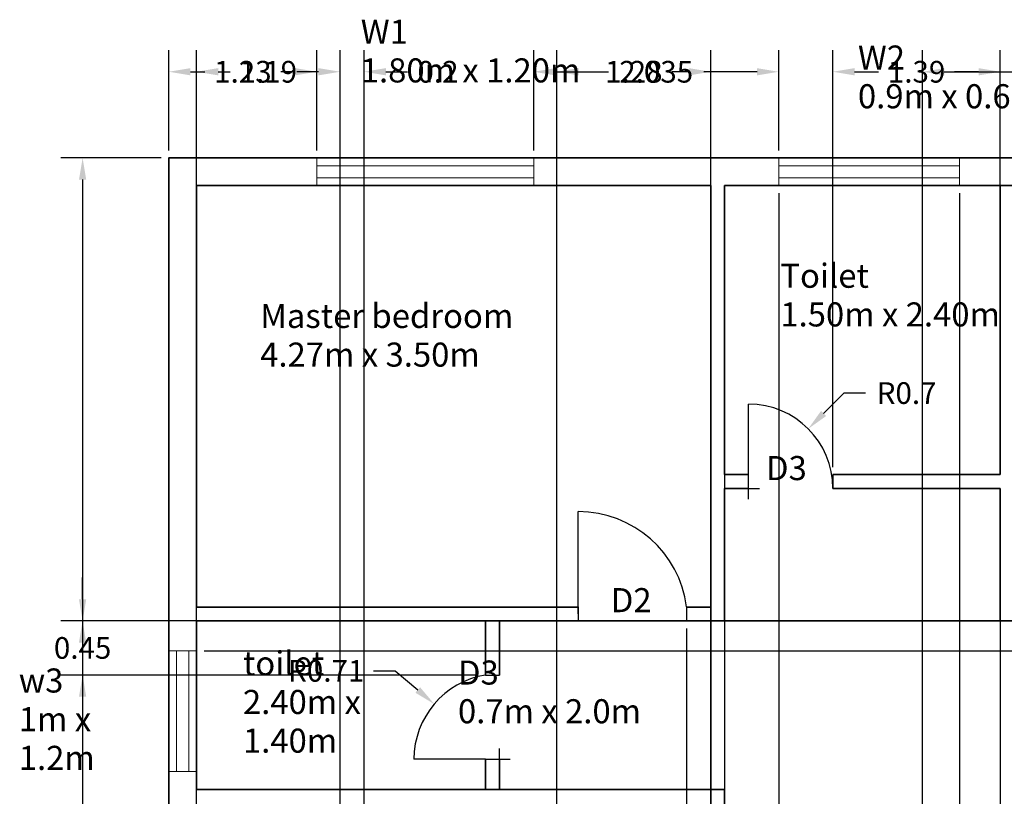
# Model space of a CAD drawing. Units: metres. Extents: x 1585.4 to 1599.4, y 2063.3 to 2076.9.
# Tile 2 of 3: x 1585.7 to 1593.9, y 2070.4 to 2076.9. Entities that reach past the tile are written whole.
import ezdxf

# ---------------------------------------------------------------- set-up
doc = ezdxf.new("R2010")
doc.units = ezdxf.units.M
for name, color, linetype, lineweight in [('A-ANNO-DIMS', 2, 'Continuous', 18), ('A-ANNO-TEXT', 7, 'Continuous', 18), ('A-AREA-IDEN', 7, 'Continuous', 18), ('A-DOOR', 3, 'Continuous', 25), ('A-GLAZ', 4, 'Continuous', 18), ('A-WALL', 7, 'Continuous', 35)]:
    doc.layers.add(name, color=color, linetype=linetype, lineweight=lineweight)
doc.styles.get("Standard").update_dxf_attribs({"font": 'arial.ttf'})
doc.dimstyles.get("Standard").update_dxf_attribs({"dimtxt": 0.18, "dimasz": 0.18, "dimexe": 0.18, "dimexo": 0.0625, "dimgap": 0.09, "dimtad": 0, "dimtih": 1, "dimtoh": 1, "dimdec": 4, "dimzin": 0, "dimdsep": 46, "dimtxsty": 'Standard', "dimcen": 0.09, "dimadec": 0, "dimazin": 0, "dimtfac": 1, "dimtdec": 4, "dimtofl": 0, "dimtmove": 0, "dimatfit": 3, "dimfxl": 1, "dimtolj": 1, "dimtzin": 0, "dimarcsym": 0})

# ---------------------------------------------------------------- blocks, each defined once
blk = doc.blocks.new('WIN-FRAME-1800')
for p, q in [((0, 0), (0, 0.23)), ((0, 0.23), (1.8, 0.23)), ((1.8, 0.23), (1.8, 0))]:
    blk.add_line(p, q)
blk = doc.blocks.new('WIN-FRAME-1500')
for p, q in [((0, 0), (0, 0.23)), ((0, 0.23), (1.5, 0.23)), ((1.5, 0.23), (1.5, 0))]:
    blk.add_line(p, q)
blk = doc.blocks.new('WIN-FRAME-1000')
for p, q in [((0, 0), (0, 1)), ((0, 1), (0.23, 1)), ((0.23, 0), (0, 0))]:
    blk.add_line(p, q)
blk = doc.blocks.new('DOOR-900-JAMBS-SWING')
for p, q in [((0.7923, 0.9), (0.9073, 0.9)), ((0.7923, 0), (0.9073, 0))]:
    blk.add_line(p, q)
blk.add_arc((0.9073, 0), 0.9073, 97.28167, 180)
blk = doc.blocks.new('*D7')
at = {"layer": 'A-ANNO-DIMS', "color": 0, "lineweight": -2, "transparency": 16777216}
for p, q in [((1586.8683, 2075.7088), (1586.0348, 2075.7088)), ((1586.2148, 2075.5288), (1586.2148, 2070.1307)), ((1586.2148, 2064.3688), (1586.2148, 2069.7669)), ((1591.4833, 2064.1888), (1586.0348, 2064.1888))]:
    blk.add_line(p, q, dxfattribs=at)
at = {"layer": 'A-ANNO-DIMS', "color": 0, "transparency": 16777216}
for points in [[(1586.1848, 2075.5288), (1586.2448, 2075.5288), (1586.2148, 2075.7088)], [(1586.1848, 2064.3688), (1586.2448, 2064.3688), (1586.2148, 2064.1888)]]:
    blk.add_solid(points, dxfattribs=at)
at = {"layer": 'Defpoints', "color": 0, "transparency": 16777216}
for p in [(1586.2148, 2075.7088), (1586.9308, 2075.7088), (1591.5458, 2064.1888)]:
    blk.add_point(p, dxfattribs=at)
at = {"layer": 'A-ANNO-DIMS', "color": 0, "transparency": 16777216, "insert": (1586.2148, 2069.9488), "char_height": 0.18, "attachment_point": 5}
blk.add_mtext('\\A1;11.52', dxfattribs=at)
blk = doc.blocks.new('*D8')
at = {"layer": 'A-ANNO-DIMS', "color": 0, "lineweight": -2, "transparency": 16777216}
for p, q in [((1590.1533, 2067.2463), (1590.1533, 2076.6048)), ((1591.4308, 2067.2463), (1591.4308, 2076.6048)), ((1590.3333, 2076.4248), (1590.4766, 2076.4248)), ((1591.2508, 2076.4248), (1591.1076, 2076.4248))]:
    blk.add_line(p, q, dxfattribs=at)
at = {"layer": 'A-ANNO-DIMS', "color": 0, "transparency": 16777216}
for points in [[(1590.3333, 2076.4548), (1590.3333, 2076.3948), (1590.1533, 2076.4248)], [(1591.2508, 2076.4548), (1591.2508, 2076.3948), (1591.4308, 2076.4248)]]:
    blk.add_solid(points, dxfattribs=at)
at = {"layer": 'Defpoints', "color": 0, "transparency": 16777216}
for p in [(1591.4308, 2076.4248), (1590.1533, 2067.1838), (1591.4308, 2067.1838)]:
    blk.add_point(p, dxfattribs=at)
at = {"layer": 'A-ANNO-DIMS', "color": 0, "transparency": 16777216, "insert": (1590.7921, 2076.4248), "char_height": 0.18, "attachment_point": 5}
blk.add_mtext('\\A1;1.28', dxfattribs=at)
blk = doc.blocks.new('*D11')
at = {"layer": 'A-ANNO-DIMS', "color": 0, "lineweight": -2, "transparency": 16777216}
for p, q in [((1586.9308, 2075.7713), (1586.9308, 2076.6048)), ((1588.1608, 2075.7713), (1588.1608, 2076.6048)), ((1587.1108, 2076.4248), (1587.2305, 2076.4248)), ((1587.9808, 2076.4248), (1587.8611, 2076.4248))]:
    blk.add_line(p, q, dxfattribs=at)
at = {"layer": 'A-ANNO-DIMS', "color": 0, "transparency": 16777216}
for points in [[(1587.1108, 2076.4548), (1587.1108, 2076.3948), (1586.9308, 2076.4248)], [(1587.9808, 2076.4548), (1587.9808, 2076.3948), (1588.1608, 2076.4248)]]:
    blk.add_solid(points, dxfattribs=at)
at = {"layer": 'Defpoints', "color": 0, "transparency": 16777216}
for p in [(1588.1608, 2076.4248), (1586.9308, 2075.7088), (1588.1608, 2075.7088)]:
    blk.add_point(p, dxfattribs=at)
at = {"layer": 'A-ANNO-DIMS', "color": 0, "transparency": 16777216, "insert": (1587.5458, 2076.4248), "char_height": 0.18, "attachment_point": 5}
blk.add_mtext('\\A1;1.23', dxfattribs=at)
blk = doc.blocks.new('*D12')
at = {"layer": 'A-ANNO-DIMS', "color": 0, "lineweight": -2, "transparency": 16777216}
for p, q in [((1589.9608, 2075.7713), (1589.9608, 2076.6048)), ((1591.9958, 2075.7713), (1591.9958, 2076.6048)), ((1590.1408, 2076.4248), (1590.5824, 2076.4248)), ((1591.8158, 2076.4248), (1591.3742, 2076.4248))]:
    blk.add_line(p, q, dxfattribs=at)
at = {"layer": 'A-ANNO-DIMS', "color": 0, "transparency": 16777216}
for points in [[(1590.1408, 2076.4548), (1590.1408, 2076.3948), (1589.9608, 2076.4248)], [(1591.8158, 2076.4548), (1591.8158, 2076.3948), (1591.9958, 2076.4248)]]:
    blk.add_solid(points, dxfattribs=at)
at = {"layer": 'Defpoints', "color": 0, "transparency": 16777216}
for p in [(1591.9958, 2076.4248), (1589.9608, 2075.7088), (1591.9958, 2075.7088)]:
    blk.add_point(p, dxfattribs=at)
at = {"layer": 'A-ANNO-DIMS', "color": 0, "transparency": 16777216, "insert": (1590.9783, 2076.4248), "char_height": 0.18, "attachment_point": 5}
blk.add_mtext('\\A1;2.035', dxfattribs=at)
blk = doc.blocks.new('*D13')
at = {"layer": 'A-ANNO-DIMS', "color": 0, "lineweight": -2, "transparency": 16777216}
for p, q in [((1591.9958, 2075.4163), (1591.9958, 2063.2928)), ((1593.4958, 2075.4163), (1593.4958, 2063.2928)), ((1592.1758, 2063.4728), (1592.4998, 2063.4728)), ((1593.3158, 2063.4728), (1592.9919, 2063.4728))]:
    blk.add_line(p, q, dxfattribs=at)
at = {"layer": 'A-ANNO-DIMS', "color": 0, "transparency": 16777216}
for points in [[(1592.1758, 2063.5028), (1592.1758, 2063.4428), (1591.9958, 2063.4728)], [(1593.3158, 2063.5028), (1593.3158, 2063.4428), (1593.4958, 2063.4728)]]:
    blk.add_solid(points, dxfattribs=at)
at = {"layer": 'Defpoints', "color": 0, "transparency": 16777216}
for p in [(1591.9958, 2075.4788), (1593.4958, 2075.4788), (1593.4958, 2063.4728)]:
    blk.add_point(p, dxfattribs=at)
at = {"layer": 'A-ANNO-DIMS', "color": 0, "transparency": 16777216, "insert": (1592.7458, 2063.4728), "char_height": 0.18, "attachment_point": 5}
blk.add_mtext('\\A1;1.5', dxfattribs=at)
blk = doc.blocks.new('*D21')
at = {"layer": 'A-ANNO-DIMS', "color": 0, "lineweight": -2, "transparency": 16777216}
for p, q in [((1598.1468, 2072.0438), (1598.1468, 2072.2238)), ((1587.2233, 2071.8638), (1598.3268, 2071.8638)), ((1587.2233, 2071.6138), (1598.3268, 2071.6138)), ((1598.1468, 2071.4338), (1598.1468, 2071.2538)), ((1598.1468, 2071.2538), (1597.9668, 2071.2538))]:
    blk.add_line(p, q, dxfattribs=at)
at = {"layer": 'A-ANNO-DIMS', "color": 0, "transparency": 16777216}
for points in [[(1598.1168, 2072.0438), (1598.1768, 2072.0438), (1598.1468, 2071.8638)], [(1598.1168, 2071.4338), (1598.1768, 2071.4338), (1598.1468, 2071.6138)]]:
    blk.add_solid(points, dxfattribs=at)
at = {"layer": 'Defpoints', "color": 0, "transparency": 16777216}
for p in [(1587.1608, 2071.8638), (1587.1608, 2071.6138), (1598.1468, 2071.6138)]:
    blk.add_point(p, dxfattribs=at)
at = {"layer": 'A-ANNO-DIMS', "color": 0, "transparency": 16777216, "insert": (1597.6424, 2071.2538), "char_height": 0.18, "attachment_point": 5}
blk.add_mtext('\\A1;0.25', dxfattribs=at)
blk = doc.blocks.new('*D22')
at = {"layer": 'A-ANNO-DIMS', "color": 0, "lineweight": -2, "transparency": 16777216}
for p, q in [((1591.4308, 2075.4163), (1591.4308, 2063.2928)), ((1591.5458, 2075.4163), (1591.5458, 2063.2928)), ((1591.2508, 2063.4728), (1591.0708, 2063.4728)), ((1591.7258, 2063.4728), (1591.9058, 2063.4728))]:
    blk.add_line(p, q, dxfattribs=at)
at = {"layer": 'A-ANNO-DIMS', "color": 0, "transparency": 16777216}
for points in [[(1591.2508, 2063.5028), (1591.2508, 2063.4428), (1591.4308, 2063.4728)], [(1591.7258, 2063.5028), (1591.7258, 2063.4428), (1591.5458, 2063.4728)]]:
    blk.add_solid(points, dxfattribs=at)
at = {"layer": 'Defpoints', "color": 0, "transparency": 16777216}
for p in [(1591.4308, 2075.4788), (1591.5458, 2075.4788), (1591.5458, 2063.4728)]:
    blk.add_point(p, dxfattribs=at)
at = {"layer": 'A-ANNO-DIMS', "color": 0, "transparency": 16777216, "insert": (1592.3002, 2063.4728), "char_height": 0.18, "attachment_point": 5}
blk.add_mtext('\\A1;0.115', dxfattribs=at)
blk = doc.blocks.new('*D23')
at = {"layer": 'A-ANNO-DIMS', "color": 0, "lineweight": -2, "transparency": 16777216}
for p, q in [((1591.5458, 2072.9013), (1591.5458, 2063.2928)), ((1593.8358, 2072.9013), (1593.8358, 2063.2928)), ((1591.7258, 2063.4728), (1592.3653, 2063.4728)), ((1593.6558, 2063.4728), (1593.0163, 2063.4728))]:
    blk.add_line(p, q, dxfattribs=at)
at = {"layer": 'A-ANNO-DIMS', "color": 0, "transparency": 16777216}
for points in [[(1591.7258, 2063.5028), (1591.7258, 2063.4428), (1591.5458, 2063.4728)], [(1593.6558, 2063.5028), (1593.6558, 2063.4428), (1593.8358, 2063.4728)]]:
    blk.add_solid(points, dxfattribs=at)
at = {"layer": 'Defpoints', "color": 0, "transparency": 16777216}
for p in [(1591.5458, 2072.9638), (1593.8358, 2072.9638), (1593.8358, 2063.4728)]:
    blk.add_point(p, dxfattribs=at)
at = {"layer": 'A-ANNO-DIMS', "color": 0, "transparency": 16777216, "insert": (1592.6908, 2063.4728), "char_height": 0.18, "attachment_point": 5}
blk.add_mtext('\\A1;2.29', dxfattribs=at)
blk = doc.blocks.new('*D26')
at = {"layer": 'A-ANNO-DIMS', "color": 0, "lineweight": -2, "transparency": 16777216}
for p, q in [((1593.1908, 2065.1163), (1593.1908, 2076.6048)), ((1597.2008, 2065.1163), (1597.2008, 2076.6048)), ((1593.3708, 2076.4248), (1594.8858, 2076.4248)), ((1597.0208, 2076.4248), (1595.5058, 2076.4248))]:
    blk.add_line(p, q, dxfattribs=at)
at = {"layer": 'A-ANNO-DIMS', "color": 0, "transparency": 16777216}
for points in [[(1593.3708, 2076.4548), (1593.3708, 2076.3948), (1593.1908, 2076.4248)], [(1597.0208, 2076.4548), (1597.0208, 2076.3948), (1597.2008, 2076.4248)]]:
    blk.add_solid(points, dxfattribs=at)
at = {"layer": 'Defpoints', "color": 0, "transparency": 16777216}
for p in [(1597.2008, 2076.4248), (1593.1908, 2065.0538), (1597.2008, 2065.0538)]:
    blk.add_point(p, dxfattribs=at)
at = {"layer": 'A-ANNO-DIMS', "color": 0, "transparency": 16777216, "insert": (1595.1958, 2076.4248), "char_height": 0.18, "attachment_point": 5}
blk.add_mtext('\\A1;4.01', dxfattribs=at)
blk = doc.blocks.new('*D27')
at = {"layer": 'A-ANNO-DIMS', "color": 0, "lineweight": -2, "transparency": 16777216}
for p, q in [((1587.1608, 2067.2463), (1587.1608, 2076.6048)), ((1588.3533, 2067.2463), (1588.3533, 2076.6048)), ((1587.3408, 2076.4248), (1587.4416, 2076.4248)), ((1588.1733, 2076.4248), (1588.0726, 2076.4248))]:
    blk.add_line(p, q, dxfattribs=at)
at = {"layer": 'A-ANNO-DIMS', "color": 0, "transparency": 16777216}
for points in [[(1587.3408, 2076.4548), (1587.3408, 2076.3948), (1587.1608, 2076.4248)], [(1588.1733, 2076.4548), (1588.1733, 2076.3948), (1588.3533, 2076.4248)]]:
    blk.add_solid(points, dxfattribs=at)
at = {"layer": 'Defpoints', "color": 0, "transparency": 16777216}
for p in [(1588.3533, 2076.4248), (1587.1608, 2067.1838), (1588.3533, 2067.1838)]:
    blk.add_point(p, dxfattribs=at)
at = {"layer": 'A-ANNO-DIMS', "color": 0, "transparency": 16777216, "insert": (1587.7571, 2076.4248), "char_height": 0.18, "attachment_point": 5}
blk.add_mtext('\\A1;1.19', dxfattribs=at)
blk = doc.blocks.new('*D28')
at = {"layer": 'A-ANNO-DIMS', "color": 0, "lineweight": -2, "transparency": 16777216}
for p, q in [((1588.3533, 2067.2463), (1588.3533, 2076.6048)), ((1588.5533, 2067.2463), (1588.5533, 2076.6048)), ((1588.1733, 2076.4248), (1587.9933, 2076.4248)), ((1588.7333, 2076.4248), (1588.9133, 2076.4248))]:
    blk.add_line(p, q, dxfattribs=at)
at = {"layer": 'A-ANNO-DIMS', "color": 0, "transparency": 16777216}
for points in [[(1588.1733, 2076.4548), (1588.1733, 2076.3948), (1588.3533, 2076.4248)], [(1588.7333, 2076.4548), (1588.7333, 2076.3948), (1588.5533, 2076.4248)]]:
    blk.add_solid(points, dxfattribs=at)
at = {"layer": 'Defpoints', "color": 0, "transparency": 16777216}
for p in [(1588.5533, 2076.4248), (1588.3533, 2067.1838), (1588.5533, 2067.1838)]:
    blk.add_point(p, dxfattribs=at)
at = {"layer": 'A-ANNO-DIMS', "color": 0, "transparency": 16777216, "insert": (1589.1663, 2076.4248), "char_height": 0.18, "attachment_point": 5}
blk.add_mtext('\\A1;0.2', dxfattribs=at)
blk = doc.blocks.new('*D31')
at = {"layer": 'A-ANNO-DIMS', "color": 0, "lineweight": -2, "transparency": 16777216}
for p, q in [((1593.8358, 2071.8013), (1593.8358, 2063.2928)), ((1594.1508, 2071.8013), (1594.1508, 2063.2928)), ((1593.6558, 2063.4728), (1593.4758, 2063.4728)), ((1594.3308, 2063.4728), (1594.5108, 2063.4728))]:
    blk.add_line(p, q, dxfattribs=at)
at = {"layer": 'A-ANNO-DIMS', "color": 0, "transparency": 16777216}
for points in [[(1593.6558, 2063.5028), (1593.6558, 2063.4428), (1593.8358, 2063.4728)], [(1594.3308, 2063.5028), (1594.3308, 2063.4428), (1594.1508, 2063.4728)]]:
    blk.add_solid(points, dxfattribs=at)
at = {"layer": 'Defpoints', "color": 0, "transparency": 16777216}
for p in [(1593.8358, 2071.8638), (1594.1508, 2071.8638), (1594.1508, 2063.4728)]:
    blk.add_point(p, dxfattribs=at)
at = {"layer": 'A-ANNO-DIMS', "color": 0, "transparency": 16777216, "insert": (1594.9052, 2063.4728), "char_height": 0.18, "attachment_point": 5}
blk.add_mtext('\\A1;0.315', dxfattribs=at)
blk = doc.blocks.new('*D32')
at = {"layer": 'A-ANNO-DIMS', "color": 0, "lineweight": -2, "transparency": 16777216}
for p, q in [((1591.4308, 2071.9163), (1591.4308, 2063.2928)), ((1591.2308, 2071.8013), (1591.2308, 2063.2928)), ((1591.0508, 2063.4728), (1590.8708, 2063.4728)), ((1591.6108, 2063.4728), (1591.7908, 2063.4728))]:
    blk.add_line(p, q, dxfattribs=at)
at = {"layer": 'A-ANNO-DIMS', "color": 0, "transparency": 16777216}
for points in [[(1591.0508, 2063.5028), (1591.0508, 2063.4428), (1591.2308, 2063.4728)], [(1591.6108, 2063.5028), (1591.6108, 2063.4428), (1591.4308, 2063.4728)]]:
    blk.add_solid(points, dxfattribs=at)
at = {"layer": 'Defpoints', "color": 0, "transparency": 16777216}
for p in [(1591.4308, 2071.9788), (1591.2308, 2071.8638), (1591.4308, 2063.4728)]:
    blk.add_point(p, dxfattribs=at)
at = {"layer": 'A-ANNO-DIMS', "color": 0, "transparency": 16777216, "insert": (1592.0438, 2063.4728), "char_height": 0.18, "attachment_point": 5}
blk.add_mtext('\\A1;0.2', dxfattribs=at)
blk = doc.blocks.new('*D34')
at = {"layer": 'A-ANNO-DIMS', "color": 0, "lineweight": -2, "transparency": 16777216}
for p, q in [((1592.4458, 2073.1413), (1592.4458, 2076.6048)), ((1593.8358, 2073.1413), (1593.8358, 2076.6048)), ((1592.6258, 2076.4248), (1592.8253, 2076.4248)), ((1593.6558, 2076.4248), (1593.4563, 2076.4248))]:
    blk.add_line(p, q, dxfattribs=at)
at = {"layer": 'A-ANNO-DIMS', "color": 0, "transparency": 16777216}
for points in [[(1592.6258, 2076.4548), (1592.6258, 2076.3948), (1592.4458, 2076.4248)], [(1593.6558, 2076.4548), (1593.6558, 2076.3948), (1593.8358, 2076.4248)]]:
    blk.add_solid(points, dxfattribs=at)
at = {"layer": 'Defpoints', "color": 0, "transparency": 16777216}
for p in [(1593.8358, 2076.4248), (1592.4458, 2073.0788), (1593.8358, 2073.0788)]:
    blk.add_point(p, dxfattribs=at)
at = {"layer": 'A-ANNO-DIMS', "color": 0, "transparency": 16777216, "insert": (1593.1408, 2076.4248), "char_height": 0.18, "attachment_point": 5}
blk.add_mtext('\\A1;1.39', dxfattribs=at)
blk = doc.blocks.new('*D35')
at = {"layer": 'A-ANNO-DIMS', "color": 0, "lineweight": -2, "transparency": 16777216}
for p, q in [((1586.214822, 2072.043841), (1586.214822, 2072.223841)), ((1589.498322, 2071.863841), (1586.034822, 2071.863841)), ((1589.498322, 2071.413841), (1586.034822, 2071.413841)), ((1586.214822, 2071.233841), (1586.214822, 2071.053841))]:
    blk.add_line(p, q, dxfattribs=at)
at = {"layer": 'A-ANNO-DIMS', "color": 0, "transparency": 16777216}
for points in [[(1586.184822, 2072.043841), (1586.244822, 2072.043841), (1586.214822, 2071.863841)], [(1586.184822, 2071.233841), (1586.244822, 2071.233841), (1586.214822, 2071.413841)]]:
    blk.add_solid(points, dxfattribs=at)
at = {"layer": 'Defpoints', "color": 0, "transparency": 16777216}
for p in [(1586.214822, 2071.863841), (1589.560822, 2071.863841), (1589.560822, 2071.413841)]:
    blk.add_point(p, dxfattribs=at)
at = {"layer": 'A-ANNO-DIMS', "color": 0, "transparency": 16777216, "insert": (1586.214822, 2071.638841), "char_height": 0.18, "attachment_point": 5}
blk.add_mtext('\\A1;0.45', dxfattribs=at)
blk = doc.blocks.new('*D36')
at = {"layer": 'A-ANNO-DIMS', "color": 0, "lineweight": -2, "transparency": 16777216}
for p, q in [((1591.5458, 2070.4013), (1591.5458, 2063.2928)), ((1597.2008, 2070.4598), (1597.2008, 2063.2928)), ((1591.7258, 2063.4728), (1593.9789, 2063.4728)), ((1597.0208, 2063.4728), (1594.7677, 2063.4728))]:
    blk.add_line(p, q, dxfattribs=at)
at = {"layer": 'A-ANNO-DIMS', "color": 0, "transparency": 16777216}
for points in [[(1591.7258, 2063.5028), (1591.7258, 2063.4428), (1591.5458, 2063.4728)], [(1597.0208, 2063.5028), (1597.0208, 2063.4428), (1597.2008, 2063.4728)]]:
    blk.add_solid(points, dxfattribs=at)
at = {"layer": 'Defpoints', "color": 0, "transparency": 16777216}
for p in [(1591.5458, 2070.4638), (1597.2008, 2070.5223), (1597.2008, 2063.4728)]:
    blk.add_point(p, dxfattribs=at)
at = {"layer": 'A-ANNO-DIMS', "color": 0, "transparency": 16777216, "insert": (1594.3733, 2063.4728), "char_height": 0.18, "attachment_point": 5}
blk.add_mtext('\\A1;5.655', dxfattribs=at)
blk = doc.blocks.new('*D37')
at = {"layer": 'A-ANNO-DIMS', "color": 0, "lineweight": -2, "transparency": 16777216}
for p, q in [((1597.1383, 2071.8638), (1586.0348, 2071.8638)), ((1586.2148, 2071.6838), (1586.2148, 2069.6)), ((1586.2148, 2067.1523), (1586.2148, 2069.2362)), ((1597.1383, 2066.9723), (1586.0348, 2066.9723))]:
    blk.add_line(p, q, dxfattribs=at)
at = {"layer": 'A-ANNO-DIMS', "color": 0, "transparency": 16777216}
for points in [[(1586.1848, 2071.6838), (1586.2448, 2071.6838), (1586.2148, 2071.8638)], [(1586.1848, 2067.1523), (1586.2448, 2067.1523), (1586.2148, 2066.9723)]]:
    blk.add_solid(points, dxfattribs=at)
at = {"layer": 'Defpoints', "color": 0, "transparency": 16777216}
for p in [(1586.2148, 2071.8638), (1597.2008, 2071.8638), (1597.2008, 2066.9723)]:
    blk.add_point(p, dxfattribs=at)
at = {"layer": 'A-ANNO-DIMS', "color": 0, "transparency": 16777216, "insert": (1586.2148, 2069.4181), "char_height": 0.18, "attachment_point": 5}
blk.add_mtext('\\A1;4.892', dxfattribs=at)
blk = doc.blocks.new('*D40')
at = {"layer": 'A-ANNO-DIMS', "color": 0, "lineweight": -2, "transparency": 16777216}
for p, q in [((1588.6306, 2071.4484), (1588.8106, 2071.4484)), ((1588.8106, 2071.4484), (1588.9978, 2071.2895)), ((1589.6758, 2070.6238), (1589.6758, 2070.8038)), ((1589.5858, 2070.7138), (1589.7658, 2070.7138))]:
    blk.add_line(p, q, dxfattribs=at)
at = {"layer": 'A-ANNO-DIMS', "color": 0, "transparency": 16777216}
blk.add_solid([(1589.0172, 2071.3123), (1588.9784, 2071.2666), (1589.135, 2071.173)], dxfattribs=at)
at = {"layer": 'Defpoints', "color": 0, "transparency": 16777216}
for p in [(1589.135, 2071.173), (1589.6758, 2070.7138)]:
    blk.add_point(p, dxfattribs=at)
at = {"layer": 'A-ANNO-DIMS', "color": 0, "transparency": 16777216, "insert": (1588.238, 2071.4484), "char_height": 0.18, "attachment_point": 5}
blk.add_mtext('\\A1;R0.71', dxfattribs=at)
blk = doc.blocks.new('*D41')
at = {"layer": 'A-ANNO-DIMS', "color": 0, "lineweight": -2, "transparency": 16777216}
for p, q in [((1592.5378, 2073.7558), (1592.3681, 2073.5861)), ((1592.7178, 2073.7558), (1592.5378, 2073.7558)), ((1591.7458, 2072.8738), (1591.7458, 2073.0538)), ((1591.6558, 2072.9638), (1591.8358, 2072.9638))]:
    blk.add_line(p, q, dxfattribs=at)
at = {"layer": 'A-ANNO-DIMS', "color": 0, "transparency": 16777216}
blk.add_solid([(1592.3469, 2073.6073), (1592.3893, 2073.5649), (1592.2408, 2073.4588)], dxfattribs=at)
at = {"layer": 'Defpoints', "color": 0, "transparency": 16777216}
for p in [(1592.2408, 2073.4588), (1591.7458, 2072.9638)]:
    blk.add_point(p, dxfattribs=at)
at = {"layer": 'A-ANNO-DIMS', "color": 0, "transparency": 16777216, "insert": (1593.0578, 2073.7558), "char_height": 0.18, "attachment_point": 5}
blk.add_mtext('\\A1;R0.7', dxfattribs=at)

msp = doc.modelspace()

# ---------------------------------------------------------------- linework, layer by layer
at = {"layer": 'A-DOOR'}
for p, q in [((1591.7458, 2073.0788), (1591.7458, 2073.6638)), ((1591.7458, 2072.9638), (1591.7458, 2073.0788)), ((1592.4458, 2073.0788), (1592.4458, 2072.9638)), ((1590.3308, 2071.9213), (1590.3308, 2072.7712)), ((1589.5608, 2071.4138), (1589.6758, 2071.4138)), ((1589.5608, 2070.7138), (1588.9664, 2070.7138)), ((1589.5608, 2070.7138), (1589.6758, 2070.7138))]:
    msp.add_line(p, q, dxfattribs=at)
for centre, radius, start, end in [((1591.7458, 2072.9638), 0.7, 360, 90), ((1589.6758, 2070.7138), 0.7094, 99.32954, 180)]:
    msp.add_arc(centre, radius, start, end, dxfattribs=at)
at = {"layer": 'A-GLAZ'}
for p, q in [((1588.1608, 2075.6438), (1589.9608, 2075.6438)), ((1591.9958, 2075.6438), (1593.4958, 2075.6438)), ((1588.1608, 2075.5438), (1589.9608, 2075.5438)), ((1591.9958, 2075.5438), (1593.4958, 2075.5438)), ((1586.9958, 2071.6138), (1586.9958, 2070.6138)), ((1587.0958, 2071.6138), (1587.0958, 2070.6138))]:
    msp.add_line(p, q, dxfattribs=at)
at = {"layer": 'A-WALL'}
for p, q in [((1586.9308, 2075.7088), (1587.1608, 2075.7088)), ((1587.1608, 2075.4788), (1591.4308, 2075.4788)), ((1587.1608, 2071.9788), (1587.1608, 2075.4788)), ((1587.1608, 2075.4788), (1588.1608, 2075.4788)), ((1591.4308, 2075.4788), (1591.4308, 2071.9788)), ((1591.5458, 2075.4788), (1591.5458, 2073.0788)), ((1591.5458, 2075.4788), (1593.8358, 2075.4788)), ((1591.5458, 2075.4788), (1591.9958, 2075.4788)), ((1593.9508, 2075.4788), (1593.8358, 2075.4788)), ((1593.8358, 2075.4788), (1593.8358, 2073.0788)), ((1591.7458, 2073.0788), (1591.5458, 2073.0788)), ((1593.8358, 2073.0788), (1592.4458, 2073.0788)), ((1591.5458, 2072.9638), (1591.7458, 2072.9638)), ((1591.5458, 2072.9638), (1591.5458, 2071.9788)), ((1591.5458, 2072.9638), (1591.7458, 2072.9638)), ((1592.4458, 2072.9638), (1593.8358, 2072.9638)), ((1593.8358, 2072.9638), (1593.8358, 2071.9788)), ((1590.3308, 2071.9788), (1587.1608, 2071.9788)), ((1591.4308, 2071.9788), (1591.2308, 2071.9788)), ((1591.4308, 2071.9788), (1591.2308, 2071.9788)), ((1591.5458, 2071.9788), (1591.5458, 2071.8638)), ((1593.8358, 2071.9788), (1593.8358, 2071.8638)), ((1587.1608, 2071.8638), (1587.1608, 2070.4638)), ((1590.3308, 2071.8638), (1587.1608, 2071.8638)), ((1589.5608, 2071.4138), (1589.5608, 2071.8638)), ((1589.6758, 2071.4138), (1589.6758, 2071.8638)), ((1591.5458, 2071.8638), (1591.2308, 2071.8638)), ((1593.8358, 2071.8638), (1594.1508, 2071.8638)), ((1589.5608, 2070.4638), (1589.5608, 2070.7138)), ((1589.6758, 2070.7138), (1589.6758, 2070.4638)), ((1587.1608, 2070.4638), (1587.1608, 2070.6138)), ((1587.1608, 2070.4638), (1589.5608, 2070.4638)), ((1589.5608, 2070.4638), (1591.4308, 2070.4638)), ((1591.4308, 2070.4638), (1591.5458, 2070.4638)), ((1591.5458, 2070.4638), (1591.5458, 2068.1988))]:
    msp.add_line(p, q, dxfattribs=at)
msp.add_lwpolyline([(1597.4308, 2064.9388), (1597.4308, 2075.7088), (1586.9308, 2075.7088), (1586.9308, 2064.9388)], dxfattribs=at)

# ---------------------------------------------------------------- block references
at = {"layer": 'A-DOOR', "rotation": 270.0000000000296}
msp.add_blockref('DOOR-900-JAMBS-SWING', (1590.3308, 2072.7712), dxfattribs=at)
at = {"layer": 'A-GLAZ'}
for name, p in [('WIN-FRAME-1800', (1588.1608, 2075.4788)), ('WIN-FRAME-1500', (1591.9958, 2075.4788)), ('WIN-FRAME-1000', (1586.9308, 2070.6138))]:
    msp.add_blockref(name, p, dxfattribs=at)

# ---------------------------------------------------------------- texts
at = {"layer": 'A-ANNO-TEXT'}
for s, p in [('W1', (1588.5249, 2076.6573)), ('W2', (1592.6536, 2076.4427)), ('1.80m x 1.20m', (1588.5249, 2076.3361)), ('0.9m x 0.60m', (1592.6536, 2076.1214)), ('D3', (1591.8899, 2073.0328)), ('D2', (1590.6012, 2071.9359)), ('D3', (1589.3319, 2071.3343)), ('w3', (1585.685, 2071.2682)), ('0.7m x 2.0m', (1589.3319, 2071.013)), ('1m x', (1585.685, 2070.9469)), ('1.2m', (1585.685, 2070.6257))]:
    msp.add_text(s, height=0.2, dxfattribs=at).set_placement(p)
at = {"layer": 'A-AREA-IDEN'}
for s, p in [('Toilet', (1592.0093, 2074.6305)), ('Master bedroom', (1587.6896, 2074.2966)), ('1.50m x 2.40m', (1592.0093, 2074.3092)), ('4.27m x 3.50m', (1587.6896, 2073.9753)), ('toilet', (1587.5465, 2071.4113)), ('2.40m x ', (1587.5465, 2071.09)), ('1.40m', (1587.5465, 2070.7687))]:
    msp.add_text(s, height=0.2, dxfattribs=at).set_placement(p)

# ---------------------------------------------------------------- dimensions: what is measured, and where the dimension line sits
at = {"layer": 'A-ANNO-DIMS'}
for base, p1, p2, override, picture, middle in [((1588.1608, 2076.4248), (1586.9308, 2075.7088), (1588.1608, 2075.7088), {"dimdec": 2, "dimlfac": 1, "dimrnd": 0, "dimzin": 0, "dimdsep": 46, "dimlunit": 2}, '*D11', (1587.5458, 2076.4248)), ((1588.3533, 2076.4248), (1587.1608, 2067.1838), (1588.3533, 2067.1838), {"dimdec": 2, "dimlfac": 1, "dimrnd": 0, "dimzin": 0, "dimdsep": 46, "dimlunit": 2}, '*D27', (1587.7571, 2076.4248)), ((1588.5533, 2076.4248), (1588.3533, 2067.1838), (1588.5533, 2067.1838), {"dimdec": 1, "dimlfac": 1, "dimrnd": 0, "dimzin": 0, "dimdsep": 46, "dimlunit": 2}, '*D28', (1589.1663, 2076.4248)), ((1591.9958, 2076.4248), (1589.9608, 2075.7088), (1591.9958, 2075.7088), {"dimdec": 3, "dimlfac": 1, "dimrnd": 0, "dimzin": 0, "dimdsep": 46, "dimlunit": 2}, '*D12', (1590.9783, 2076.4248)), ((1591.4308, 2076.4248), (1590.1533, 2067.1838), (1591.4308, 2067.1838), {"dimdec": 2, "dimlfac": 1, "dimrnd": 0, "dimzin": 0, "dimdsep": 46, "dimlunit": 2}, '*D8', (1590.7921, 2076.4248)), ((1593.8358, 2076.4248), (1592.4458, 2073.0788), (1593.8358, 2073.0788), {"dimdec": 2, "dimlfac": 1, "dimrnd": 0, "dimzin": 0, "dimdsep": 46, "dimlunit": 2}, '*D34', (1593.1408, 2076.4248)), ((1597.2008, 2076.4248), (1593.1908, 2065.0538), (1597.2008, 2065.0538), {"dimdec": 2, "dimlfac": 1, "dimrnd": 0, "dimzin": 0, "dimdsep": 46, "dimlunit": 2}, '*D26', (1595.1958, 2076.4248)), ((1591.5458, 2063.4728), (1591.4308, 2075.4788), (1591.5458, 2075.4788), {"dimdec": 3, "dimlfac": 1, "dimrnd": 0, "dimzin": 0, "dimdsep": 46, "dimlunit": 2}, '*D22', (1592.3002, 2063.4728)), ((1593.4958, 2063.4728), (1591.9958, 2075.4788), (1593.4958, 2075.4788), {"dimdec": 1, "dimlfac": 1, "dimrnd": 0, "dimzin": 0, "dimdsep": 46, "dimlunit": 2}, '*D13', (1592.7458, 2063.4728)), ((1593.8358, 2063.4728), (1591.5458, 2072.9638), (1593.8358, 2072.9638), {"dimdec": 2, "dimlfac": 1, "dimrnd": 0, "dimzin": 0, "dimdsep": 46, "dimlunit": 2}, '*D23', (1592.6908, 2063.4728)), ((1591.4308, 2063.4728), (1591.2308, 2071.8638), (1591.4308, 2071.9788), {"dimdec": 1, "dimlfac": 1, "dimrnd": 0, "dimzin": 0, "dimdsep": 46, "dimlunit": 2}, '*D32', (1592.0438, 2063.4728)), ((1594.1508, 2063.4728), (1593.8358, 2071.8638), (1594.1508, 2071.8638), {"dimdec": 3, "dimlfac": 1, "dimrnd": 0, "dimzin": 0, "dimdsep": 46, "dimlunit": 2}, '*D31', (1594.9052, 2063.4728)), ((1597.2008, 2063.4728), (1591.5458, 2070.4638), (1597.2008, 2070.5223), {"dimdec": 3, "dimlfac": 1, "dimrnd": 0, "dimzin": 0, "dimdsep": 46, "dimlunit": 2}, '*D36', (1594.3733, 2063.4728))]:
    dim = msp.add_linear_dim(base=base, p1=p1, p2=p2, dimstyle='Standard', override=override, dxfattribs=at)
    dim.commit()
    dim.dimension.update_dxf_attribs({"geometry": picture, "text_midpoint": middle})
for base, p1, p2, override, picture, middle in [((1586.2148, 2075.7088), (1591.5458, 2064.1888), (1586.9308, 2075.7088), {"dimdec": 2, "dimlfac": 1, "dimrnd": 0, "dimzin": 0, "dimdsep": 46, "dimlunit": 2}, '*D7', (1586.2148, 2069.9488)), ((1586.2148, 2071.8638), (1589.5608, 2071.4138), (1589.5608, 2071.8638), {"dimdec": 2, "dimlfac": 1, "dimrnd": 0, "dimzin": 0, "dimdsep": 46, "dimlunit": 2}, '*D35', (1586.2148, 2071.6388)), ((1598.1468, 2071.6138), (1587.1608, 2071.8638), (1587.1608, 2071.6138), {"dimdec": 2, "dimlfac": 1, "dimrnd": 0, "dimzin": 0, "dimdsep": 46, "dimlunit": 2}, '*D21', (1597.6424, 2071.2538)), ((1586.21482, 2071.86384), (1597.20082, 2066.97232), (1597.20082, 2071.86384), {"dimdec": 3, "dimlfac": 1, "dimrnd": 0, "dimzin": 0, "dimdsep": 46, "dimlunit": 2}, '*D37', (1586.21482, 2069.41808))]:
    dim = msp.add_linear_dim(base=base, p1=p1, p2=p2, angle=90, dimstyle='Standard', override=override, dxfattribs=at)
    dim.commit()
    dim.dimension.update_dxf_attribs({"geometry": picture, "text_midpoint": middle})
for center, mpoint, override, picture, middle in [((1591.7458, 2072.9638), (1592.2408, 2073.4588), {"dimdec": 1, "dimlfac": 1, "dimrnd": 0, "dimzin": 0, "dimdsep": 46, "dimlunit": 2}, '*D41', (1593.0578, 2073.7558)), ((1589.6758, 2070.7138), (1589.135, 2071.173), {"dimdec": 2, "dimlfac": 1, "dimrnd": 0, "dimzin": 0, "dimdsep": 46, "dimlunit": 2}, '*D40', (1588.238, 2071.4484))]:
    dim = msp.add_radius_dim(center=center, mpoint=mpoint, dimstyle='Standard', override=override, dxfattribs=at)
    dim.commit()
    dim.dimension.update_dxf_attribs({"geometry": picture, "text_midpoint": middle, "dimtype": 164})

doc.saveas('drawing.dxf')
